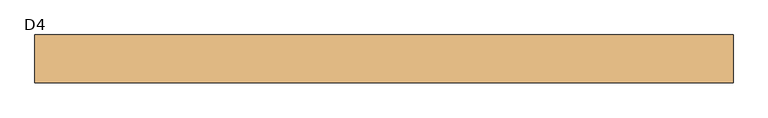
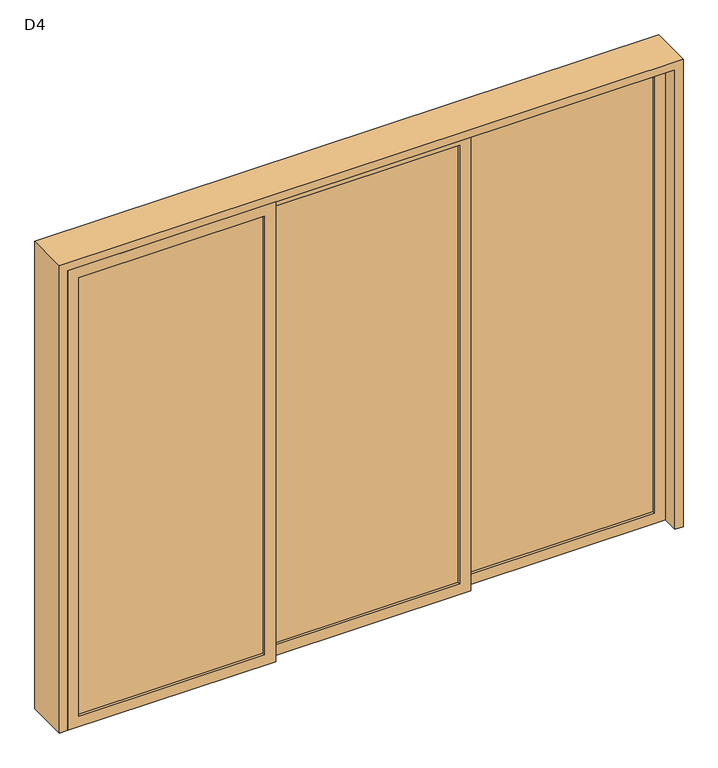
"""IFC4 building model written with IfcOpenShell, lengths in millimetres: door geometry, D4."""

from ifc_helpers import new_model, si_unit, frame, origin, place, context, project, spatial, polyline, outline, extrude, source, transform, mapped, element, save


def d4_91edf99e(model_context):
    return source(origin(), model_context, "Body", "SweptSolid", [
        extrude(outline(polyline([(1530.7580012, 1.6666667), (1530.7580012, -11.6666667), (613.2580012, -11.6666667), (613.2580012, 1.6666667), (1530.7580012, 1.6666667)])), frame((0.0, 0.0, 55.0), z_axis=(0.0, 0.0, 1.0), x_axis=(1.0, 0.0, 0.0)), (0.0, 0.0, 1.0), 2290.0),
        extrude(outline(polyline([(0.0, 1585.7580012), (2400.0, 1585.7580012), (2400.0, 558.2580012), (0.0, 558.2580012), (0.0, 1585.7580012)]), holes=[polyline([(55.0, 1530.7580012), (55.0, 613.2580012), (2345.0, 613.2580012), (2345.0, 1530.7580012), (55.0, 1530.7580012)])]), frame((0.0, -25.0, 0.0), z_axis=(0.0, 1.0, 0.0), x_axis=(0.0, 0.0, 1.0)), (0.0, 0.0, 1.0), 40.0),
        extrude(outline(polyline([(544.9246679, -38.3333333), (544.9246679, -51.6666667), (-372.5753321, -51.6666667), (-372.5753321, -38.3333333), (544.9246679, -38.3333333)])), frame((0.0, 0.0, 55.0), z_axis=(0.0, 0.0, 1.0), x_axis=(1.0, 0.0, 0.0)), (0.0, 0.0, 1.0), 2290.0),
        extrude(outline(polyline([(0.0, 599.9246679), (2400.0, 599.9246679), (2400.0, -427.5753321), (0.0, -427.5753321), (0.0, 599.9246679)]), holes=[polyline([(55.0, 544.9246679), (55.0, -372.5753321), (2345.0, -372.5753321), (2345.0, 544.9246679), (55.0, 544.9246679)])]), frame((0.0, -65.0, 0.0), z_axis=(0.0, 1.0, 0.0), x_axis=(0.0, 0.0, 1.0)), (0.0, 0.0, 1.0), 40.0),
        extrude(outline(polyline([(-441.7419988, -78.3333333), (-441.7419988, -91.6666667), (-1359.2419988, -91.6666667), (-1359.2419988, -78.3333333), (-441.7419988, -78.3333333)])), frame((0.0, 0.0, 55.0), z_axis=(0.0, 0.0, 1.0), x_axis=(1.0, 0.0, 0.0)), (0.0, 0.0, 1.0), 2290.0),
        extrude(outline(polyline([(0.0, -386.7419988), (2400.0, -386.7419988), (2400.0, -1414.2419988), (0.0, -1414.2419988), (0.0, -386.7419988)]), holes=[polyline([(55.0, -441.7419988), (55.0, -1359.2419988), (2345.0, -1359.2419988), (2345.0, -441.7419988), (55.0, -441.7419988)])]), frame((0.0, -105.0, 0.0), z_axis=(0.0, 1.0, 0.0), x_axis=(0.0, 0.0, 1.0)), (0.0, 0.0, 1.0), 40.0),
        extrude(outline(polyline([(0.0, -1454.2419988), (0.0, -1414.2419988), (2400.0, -1414.2419988), (2400.0, 1585.7580012), (0.0, 1585.7580012), (0.0, 1625.7580012), (2440.0, 1625.7580012), (2440.0, -1454.2419988), (0.0, -1454.2419988)])), frame((0.0, -105.0, 0.0), z_axis=(0.0, 1.0, 0.0), x_axis=(0.0, 0.0, 1.0)), (0.0, 0.0, 1.0), 210.0),
    ])


if __name__ == "__main__":
    model = new_model("IFC4")
    model_context = context("Model", 3, world=origin())
    ifc_project = project(units=[si_unit("LENGTHUNIT", "METRE", prefix="MILLI")], contexts=[model_context])
    site = spatial("IfcSite", under=ifc_project)
    building = spatial("IfcBuilding", under=site)
    placement = place(None, origin())
    d4_shape = d4_91edf99e(model_context)
    element("IfcDoor", 1, ObjectType="D4", at=placement, inside=building, context=model_context, shape_type="MappedRepresentation", body=[
        mapped(d4_shape, transform((0.0, 0.0, 0.0), x_axis=(1.0, 0.0, 0.0), y_axis=(0.0, 1.0, 0.0), z_axis=(0.0, 0.0, 1.0))),
    ])
    save(model, "model.ifc")

# Revit data of these elements
# Type "D4"
#   Type Mark = "59"
#   Operation = "UserDefined"
#   Width = 3000 mm
#   Thickness = 40 mm
#   Rough Width = 3080 mm
#   Rough Height = 2440 mm
#   Panel Width = 1027.5 mm
#   Panel Frame = 55 mm
#   Height = 2400 mm
#   Frame Depth = 40 mm
#   Glass Material = Sliding Door Glass
#   Frame Material = Sliding Door Frame
#   Function = (empty or 0)
# Element 1 (IfcDoor, "D4")
#   Materials on its faces: "Sliding Door Frame", "Sliding Door Glass"
# Materials
#   "Sliding Door Glass": colour RGB 247 247 247, transparency 0.68
#   "Sliding Door Frame": colour RGB 160 107 8, transparency 0
